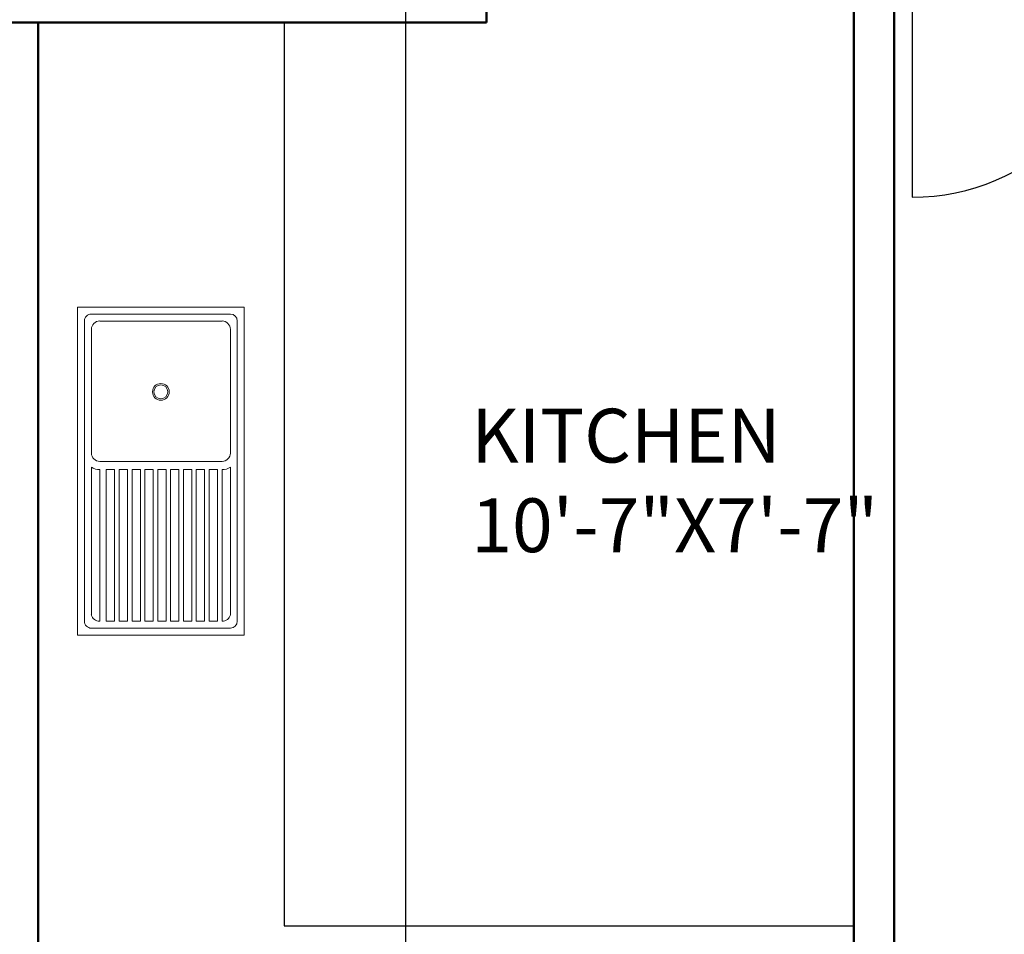
# Model space of a CAD drawing. Units: inches. Extents: x -173 to 545, y -746 to 104.
# Tile 13 of 32: x 263 to 373, y -663 to -561. Entities that reach past the tile are written whole.
import ezdxf

# ---------------------------------------------------------------- set-up
doc = ezdxf.new("R2010")
doc.units = ezdxf.units.IN
doc.header["$MEASUREMENT"] = 0
for name, color, linetype, lineweight in [('A-ANNO-DIMS', 2, 'Continuous', 18), ('A-AREA-IDEN', 7, 'Continuous', 18), ('A-DOOR', 4, 'Continuous', 25), ('A-FLOR-CASE', 9, 'Continuous', 25), ('A-FLOR-FIXT', 8, 'Continuous', 18), ('A-WALL', 7, 'Continuous', 50)]:
    doc.layers.add(name, color=color, linetype=linetype, lineweight=lineweight)
doc.styles.get("Standard").update_dxf_attribs({"font": 'arial.ttf'})
doc.dimstyles.get("Standard").update_dxf_attribs({"dimtxt": 0.18, "dimasz": 0.18, "dimexe": 0.18, "dimexo": 0.0625, "dimgap": 0.09, "dimtad": 0, "dimtih": 1, "dimtoh": 1, "dimdec": 0, "dimzin": 0, "dimdsep": 46, "dimlunit": 3, "dimtxsty": 'Standard', "dimcen": 0.09, "dimadec": 0, "dimazin": 0, "dimtfac": 1, "dimtdec": 0, "dimtofl": 0, "dimtmove": 0, "dimatfit": 3, "dimfxl": 1, "dimtolj": 1, "dimtzin": 0, "dimarcsym": 0})

# ---------------------------------------------------------------- blocks, each defined once
blk = doc.blocks.new('М11 540х1060')
for p, q in [((-1062, 540), (0, 540)), ((-1062, 0), (-1062, 540)), ((-1017, 517.5), (-45, 517.5)), ((0, 540), (0, 0)), ((-1039.5, 45), (-1039.5, 495)), ((-990, 495), (-589.5, 495)), ((-543.7, 495), (-64.8, 495)), ((-22.5, 495), (-22.5, 45)), ((-1017, 72), (-1017, 468)), ((-562.5, 72), (-562.5, 468)), ((-535.7, 468), (-45, 468)), ((-535.7, 453.4), (-45, 453.4)), ((-535.7, 453.4), (-535.7, 426.4)), ((-45, 469.5), (-45, 468)), ((-45, 453.4), (-45, 426.4)), ((-535.7, 426.4), (-45, 426.4)), ((-535.7, 411.8), (-535.7, 384.8)), ((-535.7, 411.8), (-45, 411.8)), ((-535.7, 384.8), (-45, 384.8)), ((-45, 411.8), (-45, 384.8)), ((-535.7, 370.1), (-535.7, 343.1)), ((-535.7, 370.1), (-45, 370.1)), ((-45, 370.1), (-45, 343.1)), ((-535.7, 343.1), (-45, 343.1)), ((-535.7, 328.5), (-535.7, 301.5)), ((-535.7, 328.5), (-45, 328.5)), ((-45, 328.5), (-45, 301.5)), ((-535.7, 301.5), (-45, 301.5)), ((-535.7, 286.9), (-535.7, 259.9)), ((-535.7, 286.9), (-45, 286.9)), ((-535.7, 259.9), (-45, 259.9)), ((-45, 286.9), (-45, 259.9)), ((-535.7, 245.3), (-535.7, 218.3)), ((-535.7, 245.3), (-45, 245.3)), ((-45, 245.3), (-45, 218.3)), ((-535.7, 218.3), (-45, 218.3)), ((-535.7, 203.6), (-535.7, 176.6)), ((-535.7, 203.6), (-45, 203.6)), ((-45, 203.6), (-45, 176.6)), ((-535.7, 176.6), (-45, 176.6)), ((-535.7, 162), (-45, 162)), ((-535.7, 162), (-535.7, 135)), ((-45, 162), (-45, 135)), ((-535.7, 135), (-45, 135)), ((-535.7, 120.4), (-45, 120.4)), ((-535.7, 120.4), (-535.7, 93.4)), ((-45, 120.4), (-45, 93.4)), ((-535.7, 93.4), (-45, 93.4)), ((-535.7, 72), (-45, 72)), ((-535.7, 72), (-535.7, 67.5)), ((-45, 70.5), (-45, 72)), ((-589.5, 45), (-990, 45)), ((-543.7, 45), (-64.8, 45)), ((0, 0), (-1062, 0)), ((-45, 22.5), (-1017, 22.5))]:
    blk.add_line(p, q)
for centre, major_axis, start_param, end_param in [((-1017, 495), (-15.9, 15.9), -0.785398, 0.785398), ((-45, 495), (15.9, 15.9), 5.497787, 7.068583), ((-990, 468), (19.1, 19.1), 0.785398, 2.356194), ((-589.5, 468), (-19.1, 19.1), 3.926991, 5.497787), ((-585.2, 468), (-35, 35), 3.926991, 4.503922), ((-72.3, 468.8), (-19.3, 19.3), 3.899365, 5.250385), ((-787.5, 270), (-19.1, 19.1), 3.926991, 10.210176), ((-787.5, 270), (-15.9, 15.9), 3.926991, 10.210176), ((-990, 72), (-19.1, 19.1), 0.785398, 2.356194), ((-589.5, 72), (19.1, 19.1), 3.926991, 5.497787), ((-585.2, 72), (35, 35), 4.920856, 5.497787), ((-72.3, 71.2), (19.3, 19.3), 4.174393, 5.525413), ((-1017, 45), (15.9, 15.9), 2.356194, 3.926991), ((-45, 45), (-15.9, 15.9), 2.356194, 3.926991)]:
    blk.add_ellipse(centre, major_axis=major_axis, ratio=1, start_param=start_param, end_param=end_param)
blk = doc.blocks.new('DOOR-24')
blk.add_line((24, 0), (24, 24))
blk.add_arc((24, 0), 24, 90, 180)
blk = doc.blocks.new('*D81')
at = {"layer": 'A-ANNO-DIMS', "color": 0, "lineweight": -2, "transparency": 16777216}
for p, q in [((219.8, -551.92), (219.8, -740.64)), ((306.3, -551.92), (306.3, -740.64)), ((219.98, -740.46), (262.51, -740.46)), ((306.12, -740.46), (263.59, -740.46))]:
    blk.add_line(p, q, dxfattribs=at)
at = {"layer": 'A-ANNO-DIMS', "color": 0, "transparency": 16777216}
for points in [[(219.98, -740.43), (219.98, -740.49), (219.8, -740.46)], [(306.12, -740.43), (306.12, -740.49), (306.3, -740.46)]]:
    blk.add_solid(points, dxfattribs=at)
at = {"layer": 'Defpoints', "color": 0, "transparency": 16777216}
for p in [(219.8, -551.86), (306.3, -551.86), (306.3, -740.46)]:
    blk.add_point(p, dxfattribs=at)
at = {"layer": 'A-ANNO-DIMS', "color": 0, "transparency": 16777216, "insert": (263.05, -740.46), "char_height": 0.18, "attachment_point": 5}
blk.add_mtext('\\A1;7\'-2 1/2"', dxfattribs=at)

msp = doc.modelspace()

# ---------------------------------------------------------------- linework, layer by layer
at = {"layer": 'A-FLOR-CASE'}
for p, q in [((292.76, -560.86), (292.76, -661.64)), ((292.76, -661.64), (356.3, -661.64))]:
    msp.add_line(p, q, dxfattribs=at)
at = {"layer": 'A-WALL'}
for p, q in [((315.3, -463.36), (315.3, -560.86)), ((356.3, -551.86), (356.3, -688.36)), ((360.8, -551.86), (360.8, -688.36)), ((210.8, -560.86), (315.3, -560.86)), ((265.3, -560.86), (265.3, -688.36))]:
    msp.add_line(p, q, dxfattribs=at)

# ---------------------------------------------------------------- block references
at = {"layer": 'A-DOOR', "rotation": 180}
msp.add_blockref('DOOR-24', (386.8, -556.36), dxfattribs=at)
at = {"layer": 'A-FLOR-FIXT', "xscale": 0.0344518369672997, "yscale": 0.0344518369672997, "zscale": 0.0344518369672997, "rotation": 270}
msp.add_blockref('М11 540х1060', (269.69, -629.21), dxfattribs=at)

# ---------------------------------------------------------------- texts
at = {"layer": 'A-AREA-IDEN', "insert": (313.62, -603.96), "char_height": 6, "attachment_point": 1}
msp.add_mtext('KITCHEN\\P10\'-7"X7\'-7"', dxfattribs=at)

# ---------------------------------------------------------------- dimensions: what is measured, and where the dimension line sits
at = {"layer": 'A-ANNO-DIMS'}
dim = msp.add_linear_dim(base=(306.3, -740.46), p1=(219.8, -551.86), p2=(306.3, -551.86), dimstyle='Standard', override={"dimdec": 1, "dimlfac": 1, "dimrnd": 0, "dimzin": 1, "dimdsep": 46, "dimlunit": 4, "dimfrac": 2}, dxfattribs=at)
dim.commit()
dim.dimension.update_dxf_attribs({"geometry": '*D81', "text_midpoint": (263.05, -740.46)})

doc.saveas('drawing.dxf')
